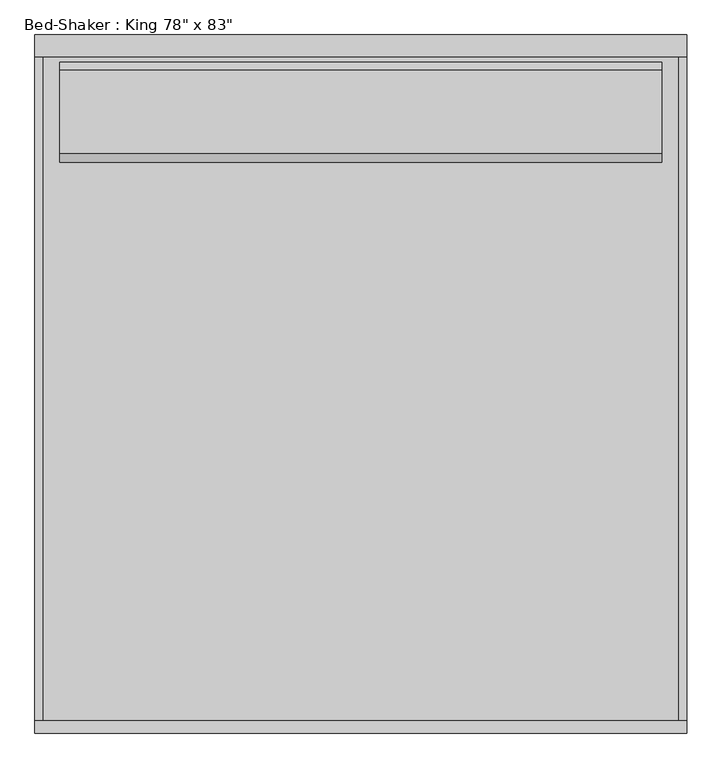
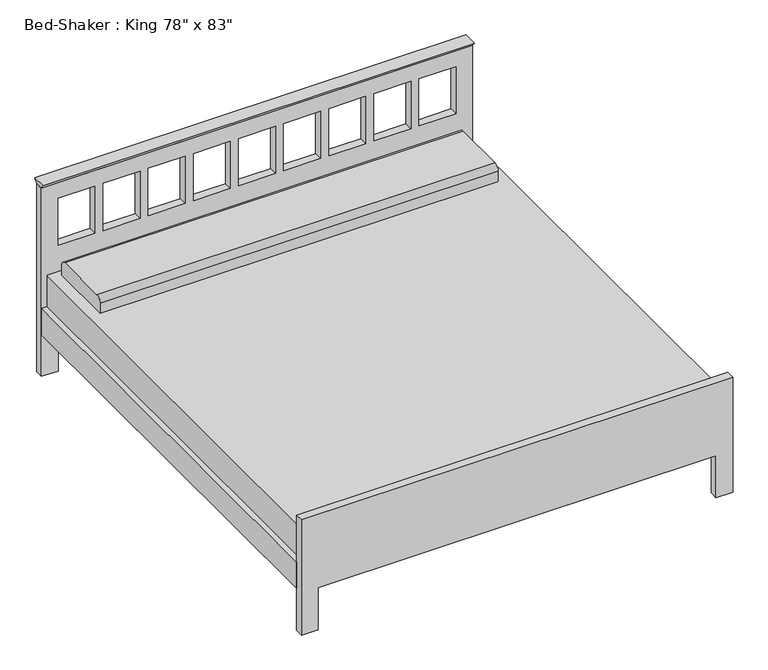
"""IFC4 building model written with IfcOpenShell, lengths in millimetres: furniture geometry."""

from ifc_helpers import new_model, si_unit, point, frame, frame_2d, origin, place, context, project, spatial, polyline, circle_curve, trimmed, segment, composite_curve, outline, extrude, source, transform, mapped, element, save


def furniture_29cd36cd(model_context):
    return source(origin(), model_context, "Body", "SweptSolid", [
        extrude(outline(polyline([(-38.1, 914.4), (-51.9545455, 933.45), (13.8545455, 933.45), (0.0, 914.4), (-38.1, 914.4)])), frame((-1009.4365546, 0.0, 0.0), z_axis=(1.0, 0.0, 0.0), x_axis=(0.0, 1.0, 0.0)), (0.0, 0.0, 1.0), 1981.2533613),
        extrude(outline(composite_curve([segment(polyline([(-373.2486637, 482.6), (-373.2486637, 533.4)]), True, "CONTINUOUS"), segment(trimmed(circle_curve(frame_2d((-347.8486637, 533.4)), 25.4), [point((-373.2486637, 533.4))], [point((-347.8486637, 558.8))], False, "CARTESIAN"), True, "CONTINUOUS"), segment(polyline([(-347.8486637, 558.8), (-93.8486637, 558.8)]), True, "CONTINUOUS"), segment(trimmed(circle_curve(frame_2d((-93.8486637, 533.4)), 25.4), [point((-93.8486637, 558.8))], [point((-68.4486637, 533.4))], False, "CARTESIAN"), True, "CONTINUOUS"), segment(polyline([(-68.4486637, 533.4), (-68.4486637, 482.6), (-373.2486637, 482.6)]), True, "CONTINUOUS")], self_intersect=False)), frame((-933.45, 0.0, 0.0), z_axis=(1.0, 0.0, 0.0), x_axis=(0.0, 1.0, 0.0)), (0.0, 0.0, 1.0), 1828.8),
        extrude(outline(polyline([(946.15, -38.1), (946.15, -2070.1), (-984.25, -2070.1), (-984.25, -38.1), (946.15, -38.1)])), frame((0.0, 0.0, 228.6), z_axis=(0.0, 0.0, 1.0), x_axis=(1.0, 0.0, 0.0)), (0.0, 0.0, 1.0), 254.0),
        extrude(outline(polyline([(946.15, -2070.1), (946.15, -38.1), (971.55, -38.1), (971.55, -2070.1), (946.15, -2070.1)])), frame((0.0, 0.0, 203.0994861), z_axis=(0.0, 0.0, 1.0), x_axis=(1.0, 0.0, 0.0)), (0.0, 0.0, 1.0), 127.0),
        extrude(outline(polyline([(-1009.65, -2070.1), (-1009.65, -38.1), (-984.25, -38.1), (-984.25, -2070.1), (-1009.65, -2070.1)])), frame((0.0, 0.0, 203.5755296), z_axis=(0.0, 0.0, 1.0), x_axis=(1.0, 0.0, 0.0)), (0.0, 0.0, 1.0), 127.0),
        extrude(outline(polyline([(0.0, -933.45), (203.2, -933.45), (203.2, 895.35), (0.0, 895.35), (0.0, 971.55), (558.8, 971.55), (558.8, -1009.65), (0.0, -1009.65), (0.0, -933.45)])), frame((0.0, -2108.2, 0.0), z_axis=(0.0, 1.0, 0.0), x_axis=(0.0, 0.0, 1.0)), (0.0, 0.0, 1.0), 38.1),
        extrude(outline(polyline([(914.4, 971.8168067), (914.4, -1009.4365546), (0.0, -1009.4365546), (0.0, -933.45), (203.2, -933.45), (203.2, 895.35), (0.0, 895.35), (0.0, 971.8168067), (914.4, 971.8168067)]), holes=[polyline([(838.2, -764.1166667), (609.6, -764.1166667), (609.6, -933.45), (838.2, -933.45), (838.2, -764.1166667)]), polyline([(838.2, -556.6833333), (609.6, -556.6833333), (609.6, -726.0166667), (838.2, -726.0166667), (838.2, -556.6833333)]), polyline([(838.2, -349.25), (609.6, -349.25), (609.6, -518.5833333), (838.2, -518.5833333), (838.2, -349.25)]), polyline([(838.2, -141.8166667), (609.6, -141.8166667), (609.6, -311.15), (838.2, -311.15), (838.2, -141.8166667)]), polyline([(838.2, 273.05), (609.6, 273.05), (609.6, 103.7166667), (838.2, 103.7166667), (838.2, 273.05)]), polyline([(838.2, 480.4833333), (609.6, 480.4833333), (609.6, 311.15), (838.2, 311.15), (838.2, 480.4833333)]), polyline([(838.2, 687.9166667), (609.6, 687.9166667), (609.6, 518.5833333), (838.2, 518.5833333), (838.2, 687.9166667)]), polyline([(838.2, 895.35), (609.6, 895.35), (609.6, 726.0166667), (838.2, 726.0166667), (838.2, 895.35)]), polyline([(838.2, 65.6166667), (609.6, 65.6166667), (609.6, -103.7166667), (838.2, -103.7166667), (838.2, 65.6166667)])]), frame((0.0, -38.1, 0.0), z_axis=(0.0, 1.0, 0.0), x_axis=(0.0, 0.0, 1.0)), (0.0, 0.0, 1.0), 38.1),
    ])


if __name__ == "__main__":
    model = new_model("IFC4")
    model_context = context("Model", 3, world=origin())
    ifc_project = project(units=[si_unit("LENGTHUNIT", "METRE", prefix="MILLI")], contexts=[model_context])
    site = spatial("IfcSite", under=ifc_project)
    building = spatial("IfcBuilding", under=site)
    placement = place(None, origin())
    furniture_shape = furniture_29cd36cd(model_context)
    element("IfcFurniture", 1, ObjectType="Bed-Shaker : King 78\" x 83\"", at=placement, inside=building, context=model_context, shape_type="MappedRepresentation", body=[
        mapped(furniture_shape, transform((0.0, 0.0, 0.0), x_axis=(1.0, 0.0, 0.0), y_axis=(0.0, 1.0, 0.0), z_axis=(0.0, 0.0, 1.0))),
    ])
    save(model, "model.ifc")

# Revit data of these elements
# Type "Bed-Shaker : King 78\" x 83\""
#   Assembly Code = "E2020200"
#   Length = 6' - 11"
#   Width = 6' - 6"
#   Frame Material = Birch
#   Mattress Material = Softwood, Lumber
#   Default Elevation = 0
# Element 1 (IfcFurniture, "Bed-Shaker : King 78\" x 83\"")
#   Materials on its faces: "Birch", "Softwood, Lumber"
# Materials
#   "Birch": class "Wood", colour RGB 210 159 95, transparency 0, Description = "Betula Alleghaniensis", Cost = 0
#   "Softwood, Lumber": class "Wood", colour RGB 223 192 134, transparency 0, Description = "Pinus Echinata", Cost = 0
